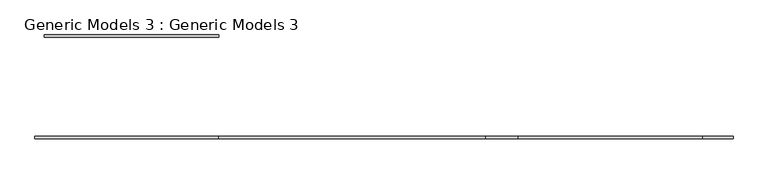
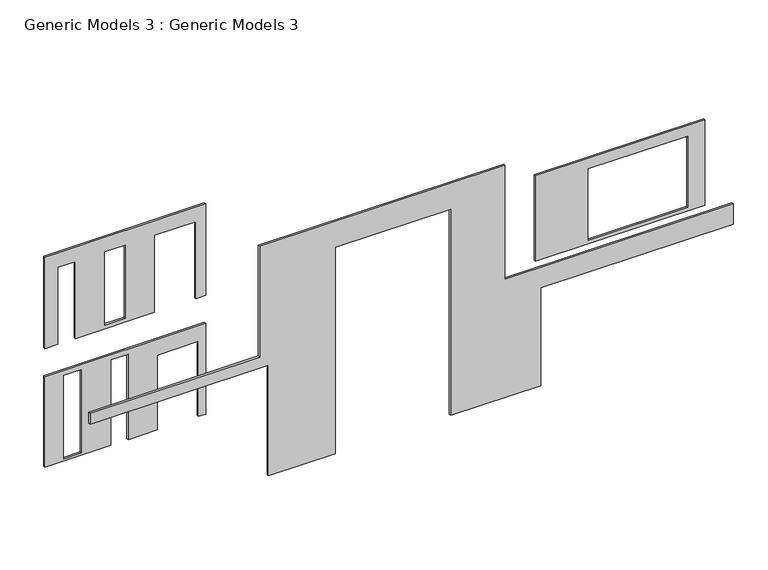
"""IFC4 building model written with IfcOpenShell, lengths in millimetres: proxy geometry, Generic Models 3 : Generic Models 3."""

from ifc_helpers import new_model, si_unit, frame, origin, place, context, project, spatial, polyline, outline, extrude, source, transform, mapped, element, save


def generic_models_3_generic_models_3_58a4acd4(model_context):
    return source(origin(), model_context, "Body", "SweptSolid", [
        extrude(outline(polyline([(5829.0338442, 13012.9903499), (5829.0338442, 8593.3903499), (3479.8, 8593.3903499), (3479.8, 13012.9903499), (5829.0338442, 13012.9903499)]), holes=[polyline([(5535.3242495, 9981.539189), (5535.3242495, 12572.339189), (3569.1752521, 12572.339189), (3569.1752521, 9981.539189), (5535.3242495, 9981.539189)])]), frame((0.0, -13427.2602599, 0.0), z_axis=(0.0, 1.0, 0.0), x_axis=(0.0, 0.0, 1.0)), (0.0, 0.0, 1.0), 50.8),
        extrude(outline(polyline([(2801.7973469, -2781.960811), (304.8, -2781.960811), (304.8, -1067.460811), (2663.3809799, -1067.460811), (2663.3809799, -610.260811), (304.8, -610.260811), (304.8, 151.739189), (2370.9547099, 151.739189), (2370.9547099, 1218.539189), (304.8, 1218.539189), (304.8, 1409.039189), (2801.7973469, 1409.039189), (2801.7973469, -2781.960811)]), holes=[polyline([(2663.3809799, -2286.660811), (2663.3809799, -1829.460811), (367.4911337, -1829.460811), (367.4911337, -2286.660811), (2663.3809799, -2286.660811)])]), frame((0.0, -10988.8602599, 0.0), z_axis=(0.0, 1.0, 0.0), x_axis=(0.0, 0.0, 1.0)), (0.0, 0.0, 1.0), 50.8),
        extrude(outline(polyline([(6096.0, 1409.039189), (6096.0, -2781.960811), (3573.1395696, -2781.960811), (3573.1395696, -2439.060811), (5692.5645868, -2439.060811), (5692.5645868, -1981.860811), (3573.1395696, -1981.860811), (3573.1395696, 75.539189), (5692.5645868, 75.539189), (5692.5645868, 1157.0058717), (3573.1395696, 1157.0058717), (3573.1395696, 1409.039189), (6096.0, 1409.039189)]), holes=[polyline([(3676.0420661, -1219.860811), (5692.5645868, -1219.860811), (5692.5645868, -686.460811), (3676.0420661, -686.460811), (3676.0420661, -1219.860811)])]), frame((0.0, -10988.8602599, 0.0), z_axis=(0.0, 1.0, 0.0), x_axis=(0.0, 0.0, 1.0)), (0.0, 0.0, 1.0), 50.8),
        extrude(outline(polyline([(3253.5878782, 7801.5944752), (6400.8, 7801.5944752), (6400.8, 1409.039189), (3352.8, 1409.039189), (3352.8, -3010.560811), (3048.0, -3010.560811), (3048.0, 1637.639189), (0.0, 1637.639189), (0.0, 3377.539189), (5689.6, 3377.539189), (5689.6, 6388.7475094), (0.0, 6388.7475094), (0.0, 8734.9360339), (2692.731124, 8734.9360339), (2692.731124, 13753.439189), (3253.5878782, 13753.439189), (3253.5878782, 7801.5944752)])), frame((0.0, -13427.2602599, 0.0), z_axis=(0.0, 1.0, 0.0), x_axis=(0.0, 0.0, 1.0)), (0.0, 0.0, 1.0), 50.8),
    ])


if __name__ == "__main__":
    model = new_model("IFC4")
    model_context = context("Model", 3, world=origin())
    ifc_project = project(units=[si_unit("LENGTHUNIT", "METRE", prefix="MILLI")], contexts=[model_context])
    site = spatial("IfcSite", under=ifc_project)
    building = spatial("IfcBuilding", under=site)
    placement = place(None, origin())
    generic_models_3_generic_models_3_shape = generic_models_3_generic_models_3_58a4acd4(model_context)
    element("IfcBuildingElementProxy", 1, Name="Generic Models 3 : Generic Models 3", ObjectType="Generic Models 3 : Generic Models 3", at=placement, inside=building, context=model_context, shape_type="MappedRepresentation", body=[
        mapped(generic_models_3_generic_models_3_shape, transform((0.0, 0.0, 0.0), x_axis=(1.0, 0.0, 0.0), y_axis=(0.0, 1.0, 0.0), z_axis=(0.0, 0.0, 1.0))),
    ])
    save(model, "model.ifc")
